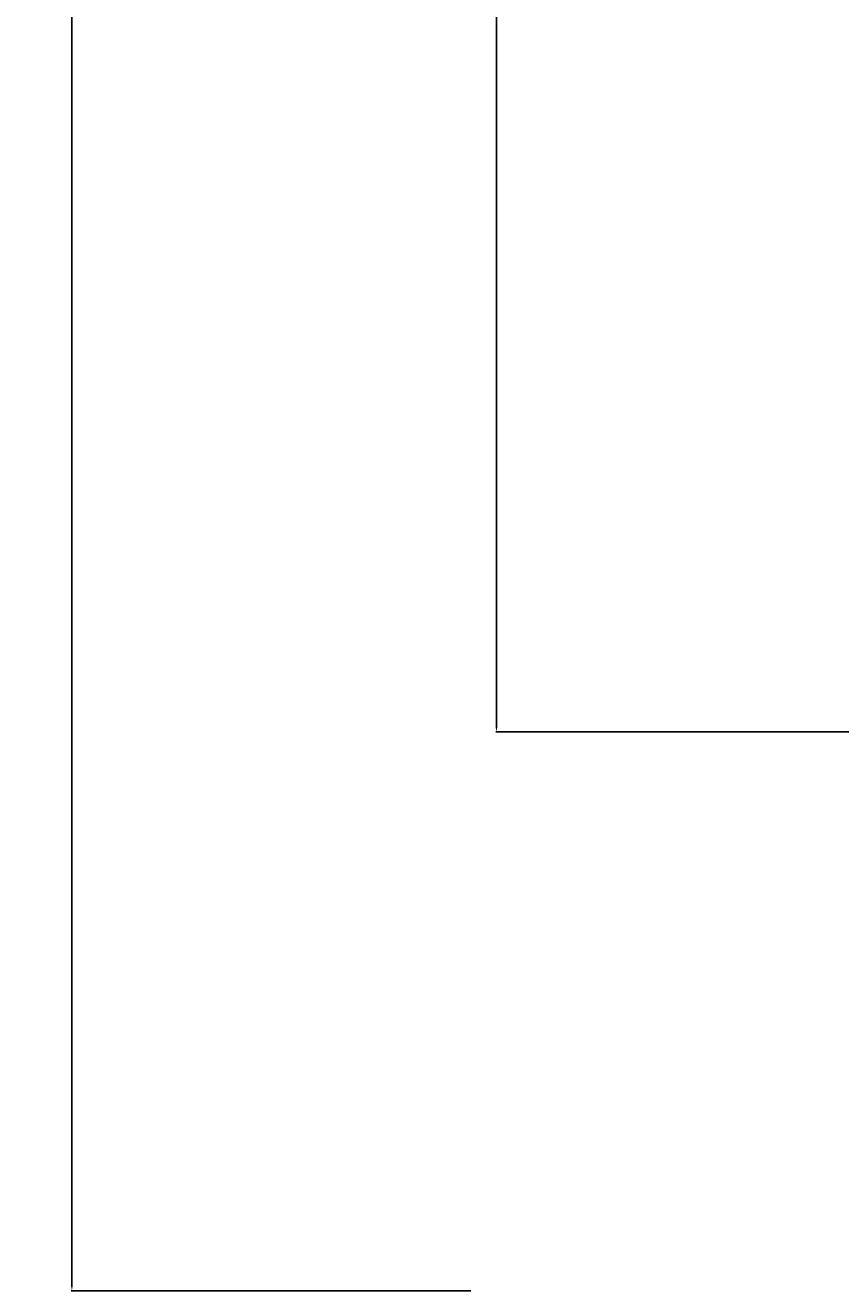
# Model space of a CAD drawing. Units: inches. Extents: x -364 to 705, y -52 to 1250.
# Tile 1 of 34: x -364 to -163, y 11 to 323. Entities that reach past the tile are written whole.
import ezdxf

# ---------------------------------------------------------------- set-up
doc = ezdxf.new("R2010")
doc.units = ezdxf.units.IN
doc.header["$MEASUREMENT"] = 0
doc.layers.add('A-ANNO-DIMS', color=4, linetype='Continuous', lineweight=18)
doc.styles.get("Standard").update_dxf_attribs({"font": 'arial.ttf'})
doc.dimstyles.get("Standard").update_dxf_attribs({"dimtxt": 1, "dimasz": 1, "dimexe": 0.18, "dimexo": 0.0625, "dimgap": 0.09, "dimtad": 0, "dimtih": 1, "dimtoh": 1, "dimdec": 0, "dimzin": 0, "dimdsep": 46, "dimlunit": 3, "dimtxsty": 'Standard', "dimcen": 0.09, "dimadec": 0, "dimazin": 0, "dimtfac": 1, "dimtdec": 0, "dimtofl": 0, "dimtmove": 0, "dimatfit": 3, "dimfxl": 1, "dimtolj": 1, "dimtzin": 0, "dimarcsym": 0})

# ---------------------------------------------------------------- blocks, each defined once
blk = doc.blocks.new('*D18')
at = {"layer": 'A-ANNO-DIMS', "color": 0, "lineweight": -2, "transparency": 16777216}
for p, q in [((-254.46, 1079.11), (-353.05, 1079.11)), ((-352.87, 1078.11), (-352.87, 551.84)), ((-352.87, 12.11), (-352.87, 538.39)), ((-254.46, 11.11), (-353.05, 11.11))]:
    blk.add_line(p, q, dxfattribs=at)
at = {"layer": 'A-ANNO-DIMS', "color": 0, "transparency": 16777216}
for points in [[(-353.04, 1078.11), (-352.7, 1078.11), (-352.87, 1079.11)], [(-353.04, 12.11), (-352.7, 12.11), (-352.87, 11.11)]]:
    blk.add_solid(points, dxfattribs=at)
at = {"layer": 'Defpoints', "color": 0, "transparency": 16777216}
for p in [(-254.4, 1079.11), (-352.87, 11.11), (-254.4, 11.11)]:
    blk.add_point(p, dxfattribs=at)
at = {"layer": 'A-ANNO-DIMS', "color": 0, "transparency": 16777216, "insert": (-352.87, 545.11), "char_height": 1, "width": 1.6985, "attachment_point": 5}
blk.add_mtext("\\A1;{\\H13x;89'}", dxfattribs=at)
blk = doc.blocks.new('*D19')
at = {"layer": 'A-ANNO-DIMS', "color": 0, "lineweight": -2, "transparency": 16777216}
for p, q in [((28.52, 986.11), (-248.33, 986.11)), ((-248.15, 985.11), (-248.15, 574.22)), ((-248.15, 149.87), (-248.15, 560.77)), ((28.52, 148.87), (-248.33, 148.87))]:
    blk.add_line(p, q, dxfattribs=at)
at = {"layer": 'A-ANNO-DIMS', "color": 0, "transparency": 16777216}
for points in [[(-248.32, 985.11), (-247.99, 985.11), (-248.15, 986.11)], [(-248.32, 149.87), (-247.99, 149.87), (-248.15, 148.87)]]:
    blk.add_solid(points, dxfattribs=at)
at = {"layer": 'Defpoints', "color": 0, "transparency": 16777216}
for p in [(28.58, 986.11), (-248.15, 148.87), (28.58, 148.87)]:
    blk.add_point(p, dxfattribs=at)
at = {"layer": 'A-ANNO-DIMS', "color": 0, "transparency": 16777216, "insert": (-248.15, 567.49), "char_height": 1, "attachment_point": 5}
blk.add_mtext('\\A1;{\\H13x;69\'-9"}', dxfattribs=at)

msp = doc.modelspace()

# ---------------------------------------------------------------- dimensions: what is measured, and where the dimension line sits
at = {"layer": 'A-ANNO-DIMS'}
for base, p1, p2, picture, middle in [((-352.87, 11.11), (-254.4, 1079.11), (-254.4, 11.11), '*D18', (-352.87, 545.11)), ((-248.15, 148.87), (28.58, 986.11), (28.58, 148.87), '*D19', (-248.15, 567.49))]:
    dim = msp.add_linear_dim(base=base, p1=p1, p2=p2, angle=90, text='{\\H13x;<>}', dimstyle='Standard', override={"dimclrd": 0, "dimclre": 0, "dimclrt": 0}, dxfattribs=at)
    dim.commit()
    dim.dimension.update_dxf_attribs({"geometry": picture, "text_midpoint": middle})

doc.saveas('drawing.dxf')
